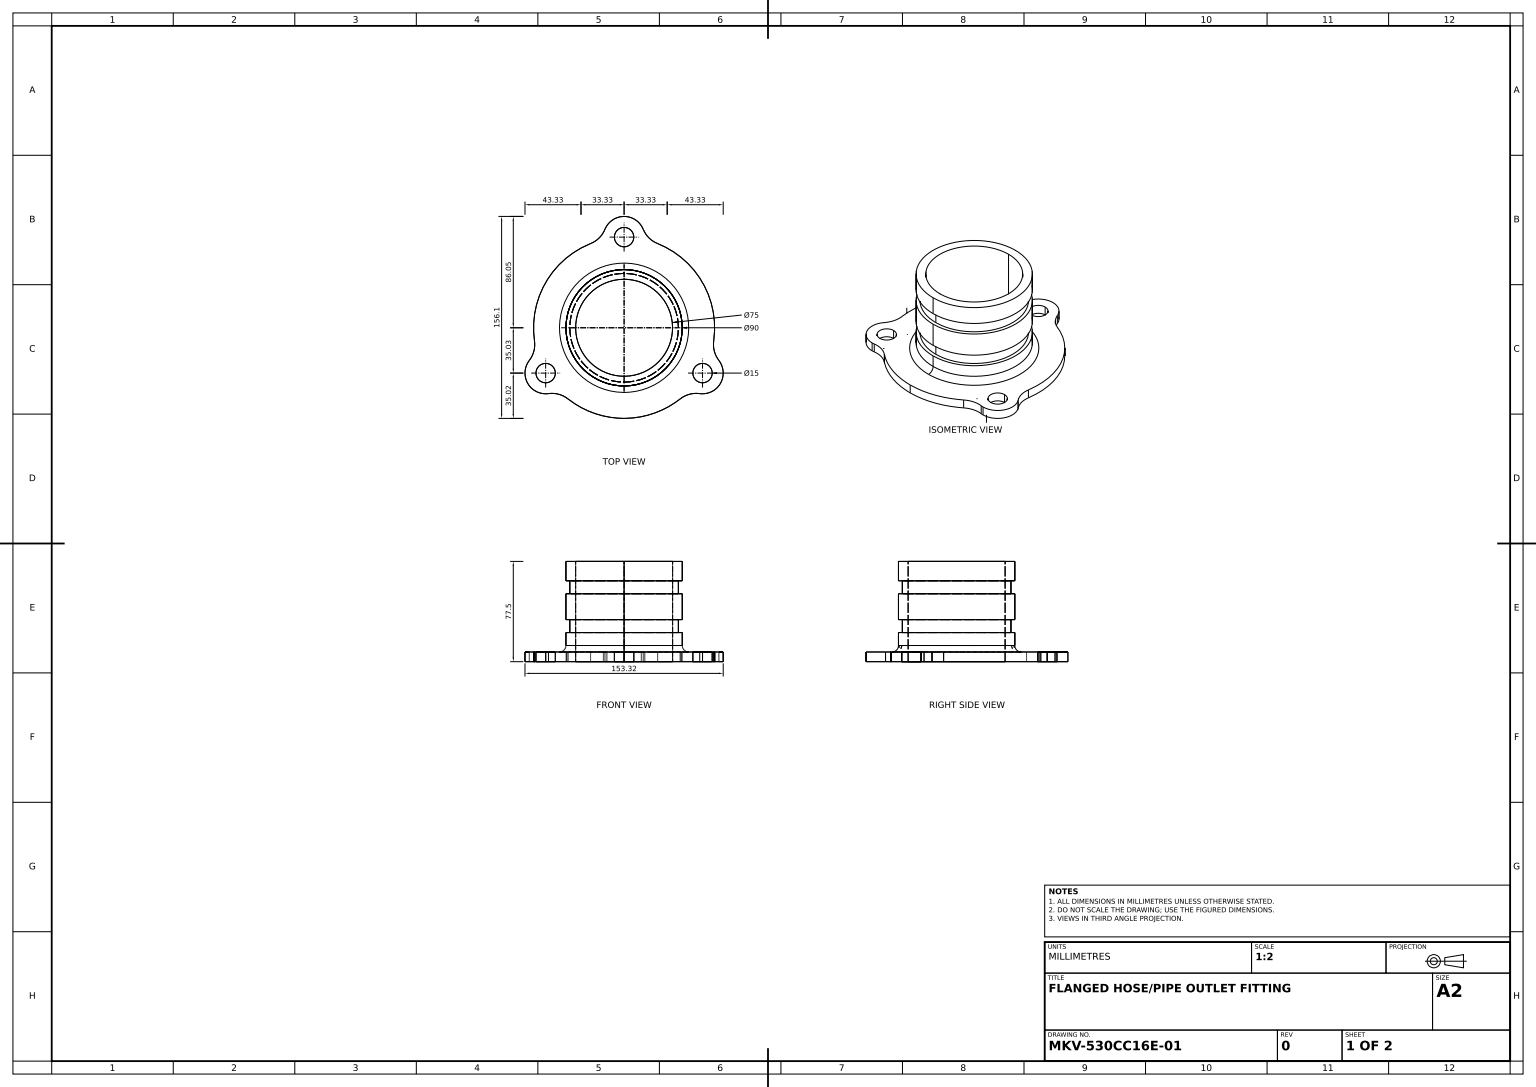
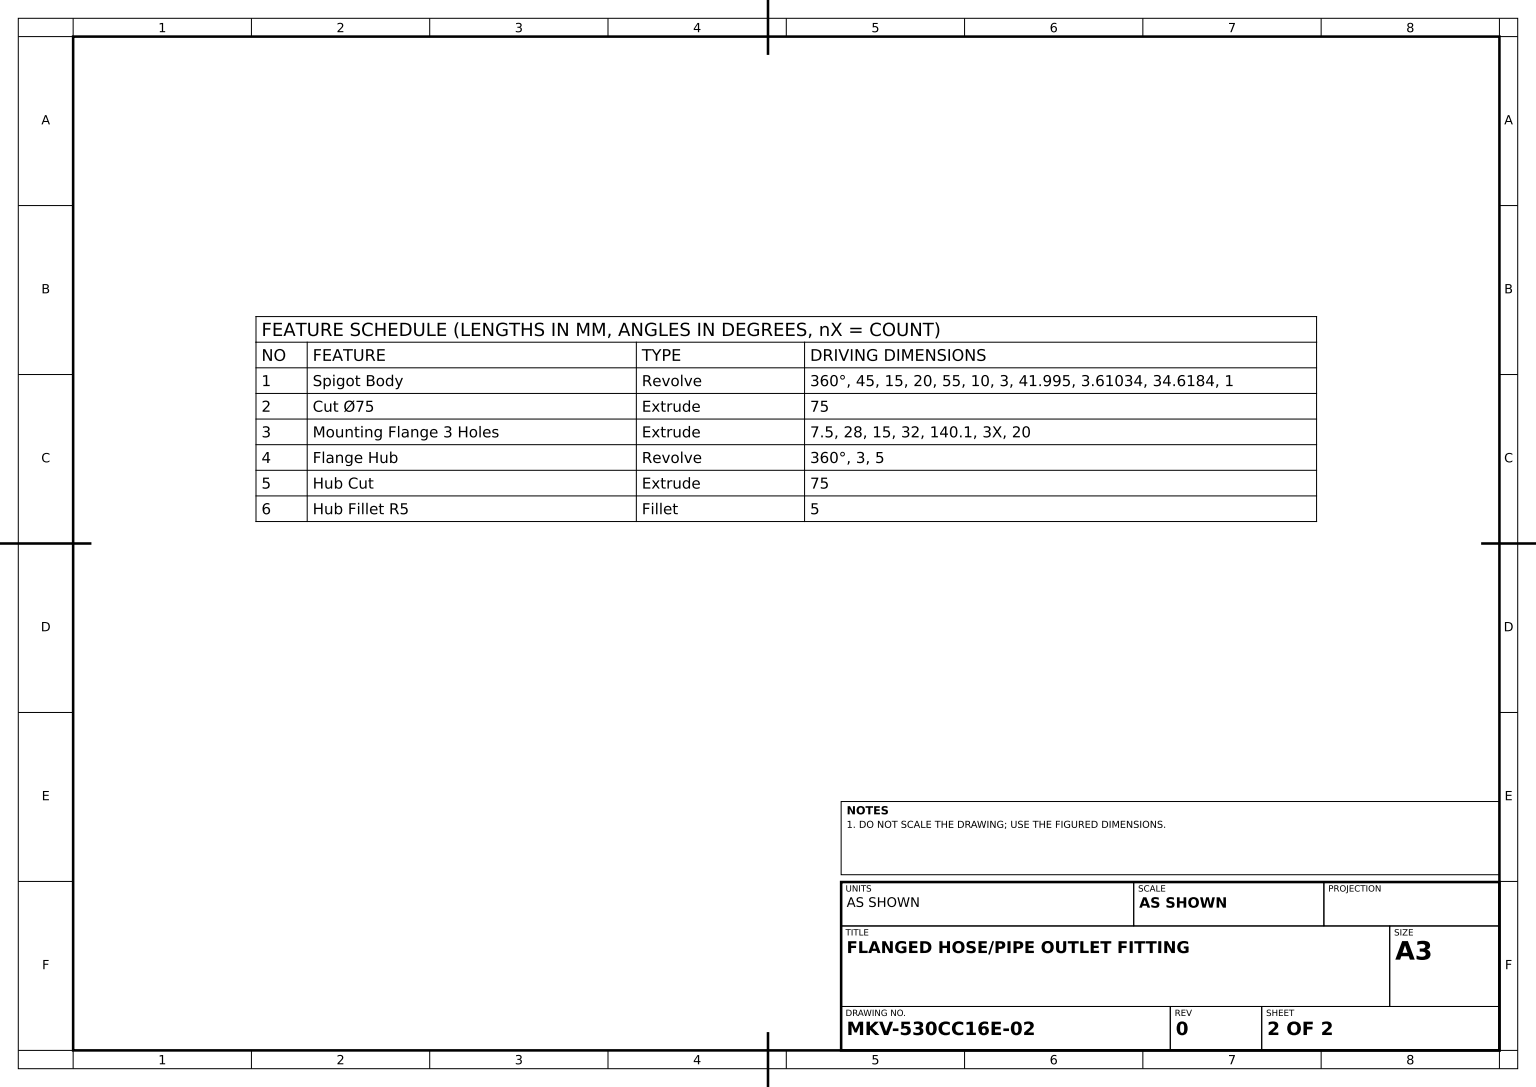
SolidWorks part; units mm, degrees
material "Plain Carbon Steel"
ref_plane "Front Plane" through (0, 0, 0) normal (0, 0, 1) x (1, 0, 0)
ref_plane "Top Plane" through (0, 0, 0) normal (0, 1, 0) x (1, 0, 0)
ref_plane "Right Plane" through (0, 0, 0) normal (1, 0, 0) x (0, 0, -1)
sketch "Spigot Profile Sketch" plane through (0, 0, 0) normal (0, 0, 1) x (1, 0, 0)
  line L0 (0, 45.6054) -> (0, -47.6233) construction
  line L1 (0, 41.995) -> (-45, 41.995)
  line L2 (-45, 41.995) -> (-45, 26.995)
  line L3 (-45, 26.995) -> (-42, 26.995)
  line L4 (-42, 26.995) -> (-42, 16.995)
  line L5 (-42, 16.995) -> (-45, 16.995)
  line L6 (-45, 16.995) -> (-45, -3.005)
  line L7 (-45, -3.005) -> (-42, -3.005)
  line L8 (-42, -3.005) -> (-42, -13.005)
  line L9 (-42, -13.005) -> (0, -13.005)
  line L10 (-42, -13.005) -> (-43, -13.005)
  dimension "D7" = 41.995
  dimension "D1" = 45
  dimension "D2" = 3
  dimension "D3" = 15
  dimension "D4" = 20
  dimension "D5" = 55
  dimension "D6" = 10
  dimension "D8" = 3.6103
  dimension "D9" = 34.6184
  dimension "D10" = 1
revolve "Spigot Body" add sketch "Spigot Profile Sketch" angle 360 about L0
sketch "Cut Circle Ø75 Sketch" plane through (0, 41.995, 0) normal (0, 1, 0) x (1, 0, 0)
  circle A0 centre (0, 0) radius 37.5
  dimension "D1" = 75
extrude "Cut Ø75" cut sketch "Cut Circle Ø75 Sketch" against normal through all
sketch "Mounting Flange Sketch" plane through (0, 0, 0) normal (0, 1, 0) x (1, 0, 0)
  line L0 (0, 0) -> (0, 54.05) construction
  line L1 (0, 62.55) -> (0, 96.8837) construction
  circle A0 centre (0, 70.05) radius 7.5
  arc A4 (14.8135, 76.0965) -> (-14.8135, 76.0965) centre (0, 70.05) ccw
  arc A6 (-64.062, -28.3384) -> (-51.135, -47.8771) centre (0, 0) ccw construction
  arc A7 (58.4947, -50.8771) -> (73.3082, -25.2194) centre (60.6651, -35.025) ccw
  circle A8 centre (60.6651, -35.025) radius 7.5
  arc A9 (-73.3082, -25.2194) -> (-58.4947, -50.8771) centre (-60.6651, -35.025) ccw
  circle A10 centre (-60.6651, -35.025) radius 7.5
  arc A11 (14.8135, 76.0965) -> (25.9278, 65.075) centre (33.3304, 83.6546) ccw
  arc A12 (-14.8135, 76.0965) -> (-25.9278, 65.075) centre (-33.3304, 83.6546) cw
  arc A13 (73.3082, -25.2194) -> (69.3205, -10.0834) centre (89.1122, -12.9623) cw
  arc A14 (58.4947, -50.8771) -> (43.3927, -54.9916) centre (55.7818, -70.6923) ccw
  arc A15 (-58.4947, -50.8771) -> (-43.3927, -54.9916) centre (-55.7818, -70.6923) cw
  arc A16 (-73.3082, -25.2194) -> (-69.3205, -10.0834) centre (-89.1122, -12.9623) ccw
  arc A17 (-43.3927, -54.9916) -> (43.3927, -54.9916) centre (0, 0) ccw
  arc A18 (-25.9278, 65.075) -> (-69.3205, -10.0834) centre (0, 0) ccw
  arc A19 (69.3205, -10.0834) -> (25.9278, 65.075) centre (0, 0) ccw
  point P8 (0, 0)
  point P16 (0, 0)
  point P36 (0, 0)
  dimension "D1" = 15
  dimension "D3" = 20
  dimension "D4" = 3
  dimension "D5" = 32
  dimension "D6" = 140.1
  dimension "D2" = 3
extrude "Mounting Flange 3 Holes" add sketch "Mounting Flange Sketch" against normal blind 7.5 from offset 28 offset against normal yes
sketch "Flange Hub Profile Sketch" plane through (0, 0, 0) normal (0, 0, 1) x (1, 0, 0)
  line L1 (58.4947, -28) -> (43.3927, -28) construction
  line L4 (-45, -28) -> (45, -28)
  line L5 (45, -28) -> (43.3927, -28)
  line L7 (-45, -28) -> (-45, -23)
  line L8 (-42, -13.005) -> (42, -13.005) construction
  line L9 (-42, -3.005) -> (-42, -13.005) construction
  line L10 (-42, -13.005) -> (42, -13.005)
  line L11 (-42, -3.005) -> (-42, -13.005)
  line L12 (-42, -13.005) -> (-45, -13.005)
  line L13 (-45, -13.005) -> (-45, -23)
  line L14 (0, 0) -> (0, -38.7997) construction
  line L15 (45, -13.005) -> (45, -23)
  line L16 (42, -13.005) -> (45, -13.005)
  line L17 (45, -23) -> (45, -28)
  dimension "D2" = 5
  dimension "D1" = 3
revolve "Flange Hub" add sketch "Flange Hub Profile Sketch" angle 360 about L14
sketch "Hub Cut Sketch" plane through (0, 41.995, 0) normal (0, 1, 0) x (1, 0, 0)
  circle A0 centre (0, 0) radius 37.5
  dimension "D1" = 75
extrude "Hub Cut" cut sketch "Hub Cut Sketch" against normal through all
fillet "Hub Fillet R5" radius 5 1 edges at (0, -28, 45)
